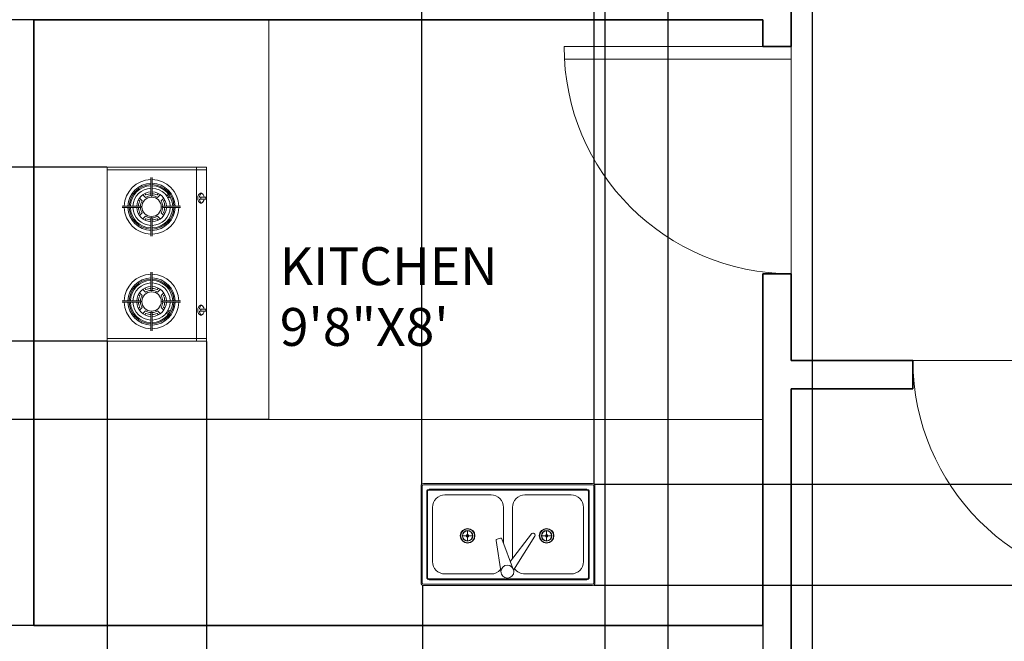
# Model space of a CAD drawing. Units: inches. Extents: x -438 to 102, y -60 to 1091.
# Tile 9 of 20: x -305 to -149, y 799 to 898. Entities that reach past the tile are written whole.
import ezdxf

# ---------------------------------------------------------------- set-up
doc = ezdxf.new("R2010")
doc.units = ezdxf.units.IN
doc.header["$MEASUREMENT"] = 0
for name, color, linetype, lineweight, true_color in [('A-ANNO-DIMS', 217, 'Continuous', 18, 0x93278f), ('A-DOOR', 30, 'Continuous', 18, 0xf26722), ('A-WALL', 2, 'Continuous', 35, 0xf1eb1f)]:
    doc.layers.add(name, color=color, linetype=linetype, lineweight=lineweight, true_color=true_color)
for name, color, linetype, lineweight in [('A-AREA-IDEN', 4, 'Continuous', 18), ('A-EQPM', 9, 'Continuous', 15), ('A-FLOR-CASE', 7, 'Continuous', 18), ('A-FLOR-FIXT', 9, 'Continuous', 15)]:
    doc.layers.add(name, color=color, linetype=linetype, lineweight=lineweight)
doc.styles.get("Standard").update_dxf_attribs({"font": 'arial.ttf'})
doc.dimstyles.get("Standard").update_dxf_attribs({"dimtxt": 8, "dimasz": 0.18, "dimexe": 0.18, "dimexo": 0.0625, "dimgap": 0.09, "dimtad": 0, "dimtih": 1, "dimtoh": 1, "dimdec": 4, "dimzin": 0, "dimdsep": 46, "dimlunit": 3, "dimtxsty": 'Standard', "dimcen": 0.09, "dimadec": 0, "dimazin": 0, "dimtfac": 1, "dimtdec": 4, "dimtofl": 0, "dimtmove": 0, "dimatfit": 3, "dimfxl": 1, "dimtolj": 1, "dimtzin": 0, "dimarcsym": 0})

# ---------------------------------------------------------------- blocks, each defined once
blk = doc.blocks.new('DOOR-SWING-36')
for p, q in [((-36, 0), (0, 0)), ((-2, 0), (-2, -36)), ((0, 0), (0, -36))]:
    blk.add_line(p, q)
blk.add_arc((0, 0), 36, 180, 270)
blk = doc.blocks.new('*D37')
at = {"layer": 'A-ANNO-DIMS', "color": 0, "lineweight": -2, "transparency": 16777216}
for p, q in [((-179.8, 234.94), (-179.8, 1079.58)), ((-134.08, 234.94), (-134.08, 1079.58)), ((-179.62, 1079.4), (-176.98, 1079.4)), ((-134.26, 1079.4), (-136.9, 1079.4))]:
    blk.add_line(p, q, dxfattribs=at)
at = {"layer": 'A-ANNO-DIMS', "color": 0, "transparency": 16777216}
for points in [[(-179.62, 1079.43), (-179.62, 1079.37), (-179.8, 1079.4)], [(-134.26, 1079.43), (-134.26, 1079.37), (-134.08, 1079.4)]]:
    blk.add_solid(points, dxfattribs=at)
at = {"layer": 'Defpoints', "color": 0, "transparency": 16777216}
for p in [(-134.08, 1079.4), (-179.8, 234.88), (-134.08, 234.88)]:
    blk.add_point(p, dxfattribs=at)
at = {"layer": 'A-ANNO-DIMS', "color": 0, "transparency": 16777216, "insert": (-156.94, 1079.4), "char_height": 8, "attachment_point": 5}
blk.add_mtext('\\A1;3\'-9 1/2"', dxfattribs=at)
blk = doc.blocks.new('*D42')
at = {"layer": 'A-ANNO-DIMS', "color": 0, "lineweight": -2, "transparency": 16777216}
for p, q in [((-266, 834.64), (-414.94, 834.64)), ((-414.76, 834.46), (-414.76, 822.55)), ((-414.76, 802.18), (-414.76, 814.09)), ((-303.21, 802), (-414.94, 802))]:
    blk.add_line(p, q, dxfattribs=at)
at = {"layer": 'A-ANNO-DIMS', "color": 0, "transparency": 16777216}
for points in [[(-414.79, 834.46), (-414.73, 834.46), (-414.76, 834.64)], [(-414.79, 802.18), (-414.73, 802.18), (-414.76, 802)]]:
    blk.add_solid(points, dxfattribs=at)
at = {"layer": 'Defpoints', "color": 0, "transparency": 16777216}
for p in [(-414.76, 834.64), (-265.94, 834.64), (-303.15, 802)]:
    blk.add_point(p, dxfattribs=at)
at = {"layer": 'A-ANNO-DIMS', "color": 0, "transparency": 16777216, "insert": (-414.76, 818.32), "char_height": 8, "attachment_point": 5}
blk.add_mtext('\\A1;2\'-8 1/2"', dxfattribs=at)
blk = doc.blocks.new('*D51')
at = {"layer": 'A-ANNO-DIMS', "color": 0, "lineweight": -2, "transparency": 16777216}
for p, q in [((-291.54, 847), (-291.54, -48.58)), ((-275.79, 847), (-275.79, -48.58)), ((-291.36, -48.4), (-275.97, -48.4)), ((-275.79, -48.4), (-275.61, -48.4))]:
    blk.add_line(p, q, dxfattribs=at)
at = {"layer": 'A-ANNO-DIMS', "color": 0, "transparency": 16777216}
for points in [[(-291.36, -48.37), (-291.36, -48.43), (-291.54, -48.4)], [(-275.97, -48.37), (-275.97, -48.43), (-275.79, -48.4)]]:
    blk.add_solid(points, dxfattribs=at)
at = {"layer": 'Defpoints', "color": 0, "transparency": 16777216}
for p in [(-291.54, 847.06), (-275.79, 847.06), (-275.79, -48.4)]:
    blk.add_point(p, dxfattribs=at)
at = {"layer": 'A-ANNO-DIMS', "color": 0, "transparency": 16777216, "insert": (-255.95, -48.4), "char_height": 8, "attachment_point": 5}
blk.add_mtext('\\A1;1\'-3 1/2"', dxfattribs=at)
blk = doc.blocks.new('*D52')
at = {"layer": 'A-ANNO-DIMS', "color": 0, "lineweight": -2, "transparency": 16777216}
for p, q in [((-291.6, 874.62), (-414.94, 874.62)), ((-414.76, 874.44), (-414.76, 865.07)), ((-414.76, 847.24), (-414.76, 856.61)), ((-291.6, 847.06), (-414.94, 847.06))]:
    blk.add_line(p, q, dxfattribs=at)
at = {"layer": 'A-ANNO-DIMS', "color": 0, "transparency": 16777216}
for points in [[(-414.79, 874.44), (-414.73, 874.44), (-414.76, 874.62)], [(-414.79, 847.24), (-414.73, 847.24), (-414.76, 847.06)]]:
    blk.add_solid(points, dxfattribs=at)
at = {"layer": 'Defpoints', "color": 0, "transparency": 16777216}
for p in [(-414.76, 874.62), (-291.54, 874.62), (-291.54, 847.06)]:
    blk.add_point(p, dxfattribs=at)
at = {"layer": 'A-ANNO-DIMS', "color": 0, "transparency": 16777216, "insert": (-414.76, 860.84), "char_height": 8, "attachment_point": 5}
blk.add_mtext('\\A1;2\'-3 1/2"', dxfattribs=at)
blk = doc.blocks.new('*D53')
at = {"layer": 'A-ANNO-DIMS', "color": 0, "lineweight": -2, "transparency": 16777216}
for p, q in [((-241.7, 824.44), (-241.7, 1079.58)), ((-214.37, 824.44), (-214.37, 1079.58)), ((-241.52, 1079.4), (-214.55, 1079.4)), ((-214.37, 1079.4), (-214.19, 1079.4))]:
    blk.add_line(p, q, dxfattribs=at)
at = {"layer": 'A-ANNO-DIMS', "color": 0, "transparency": 16777216}
for points in [[(-241.52, 1079.43), (-241.52, 1079.37), (-241.7, 1079.4)], [(-214.55, 1079.43), (-214.55, 1079.37), (-214.37, 1079.4)]]:
    blk.add_solid(points, dxfattribs=at)
at = {"layer": 'Defpoints', "color": 0, "transparency": 16777216}
for p in [(-214.37, 1079.4), (-241.7, 824.38), (-214.37, 824.38)]:
    blk.add_point(p, dxfattribs=at)
at = {"layer": 'A-ANNO-DIMS', "color": 0, "transparency": 16777216, "insert": (-194.08, 1079.4), "char_height": 8, "attachment_point": 5}
blk.add_mtext('\\A1;2\'-3 1/2"', dxfattribs=at)
blk = doc.blocks.new('*D54')
at = {"layer": 'A-ANNO-DIMS', "color": 0, "lineweight": -2, "transparency": 16777216}
for p, q in [((-214.3, 824.38), (81.43, 824.38)), ((81.25, 824.2), (81.25, 820.49)), ((81.25, 808.56), (81.25, 812.28)), ((-214.43, 808.38), (81.43, 808.38))]:
    blk.add_line(p, q, dxfattribs=at)
at = {"layer": 'A-ANNO-DIMS', "color": 0, "transparency": 16777216}
for points in [[(81.22, 824.2), (81.28, 824.2), (81.25, 824.38)], [(81.22, 808.56), (81.28, 808.56), (81.25, 808.38)]]:
    blk.add_solid(points, dxfattribs=at)
at = {"layer": 'Defpoints', "color": 0, "transparency": 16777216}
for p in [(-214.37, 824.38), (81.25, 824.38), (-214.49, 808.38)]:
    blk.add_point(p, dxfattribs=at)
at = {"layer": 'A-ANNO-DIMS', "color": 0, "transparency": 16777216, "insert": (81.25, 816.38), "char_height": 8, "attachment_point": 5}
blk.add_mtext('\\A1;1\'-4"', dxfattribs=at)
blk = doc.blocks.new('*D55')
at = {"layer": 'A-ANNO-DIMS', "color": 0, "lineweight": -2, "transparency": 16777216}
for p, q in [((-241.57, 808.32), (-241.57, -48.58)), ((-187.65, 801.94), (-187.65, -48.58)), ((-241.39, -48.4), (-225.49, -48.4)), ((-187.83, -48.4), (-203.72, -48.4))]:
    blk.add_line(p, q, dxfattribs=at)
at = {"layer": 'A-ANNO-DIMS', "color": 0, "transparency": 16777216}
for points in [[(-241.39, -48.37), (-241.39, -48.43), (-241.57, -48.4)], [(-187.83, -48.37), (-187.83, -48.43), (-187.65, -48.4)]]:
    blk.add_solid(points, dxfattribs=at)
at = {"layer": 'Defpoints', "color": 0, "transparency": 16777216}
for p in [(-241.57, 808.38), (-187.65, 802), (-187.65, -48.4)]:
    blk.add_point(p, dxfattribs=at)
at = {"layer": 'A-ANNO-DIMS', "color": 0, "transparency": 16777216, "insert": (-214.61, -48.4), "char_height": 8, "attachment_point": 5}
blk.add_mtext('\\A1;4\'-6"', dxfattribs=at)
blk = doc.blocks.new('*D56')
at = {"layer": 'A-ANNO-DIMS', "color": 0, "lineweight": -2, "transparency": 16777216}
for p, q in [((-303.21, 898), (-414.94, 898)), ((-414.76, 897.82), (-414.76, 890.54)), ((-414.76, 874.8), (-414.76, 882.08)), ((-291.6, 874.62), (-414.94, 874.62))]:
    blk.add_line(p, q, dxfattribs=at)
at = {"layer": 'A-ANNO-DIMS', "color": 0, "transparency": 16777216}
for points in [[(-414.79, 897.82), (-414.73, 897.82), (-414.76, 898)], [(-414.79, 874.8), (-414.73, 874.8), (-414.76, 874.62)]]:
    blk.add_solid(points, dxfattribs=at)
at = {"layer": 'Defpoints', "color": 0, "transparency": 16777216}
for p in [(-414.76, 898), (-303.15, 898), (-291.54, 874.62)]:
    blk.add_point(p, dxfattribs=at)
at = {"layer": 'A-ANNO-DIMS', "color": 0, "transparency": 16777216, "insert": (-414.76, 886.31), "char_height": 8, "attachment_point": 5}
blk.add_mtext('\\A1;1\'-11 1/2"', dxfattribs=at)
blk = doc.blocks.new('*D61')
at = {"layer": 'A-ANNO-DIMS', "color": 0, "lineweight": -2, "transparency": 16777216}
for p, q in [((-212.65, 534.56), (-212.65, 1079.58)), ((-202.65, 534.56), (-202.65, 1079.58)), ((-212.65, 1079.4), (-212.83, 1079.4)), ((-202.83, 1079.4), (-212.47, 1079.4))]:
    blk.add_line(p, q, dxfattribs=at)
at = {"layer": 'A-ANNO-DIMS', "color": 0, "transparency": 16777216}
for points in [[(-212.47, 1079.43), (-212.47, 1079.37), (-212.65, 1079.4)], [(-202.83, 1079.43), (-202.83, 1079.37), (-202.65, 1079.4)]]:
    blk.add_solid(points, dxfattribs=at)
at = {"layer": 'Defpoints', "color": 0, "transparency": 16777216}
for p in [(-212.65, 1079.4), (-212.65, 534.5), (-202.65, 534.5)]:
    blk.add_point(p, dxfattribs=at)
at = {"layer": 'A-ANNO-DIMS', "color": 0, "transparency": 16777216, "insert": (-226.66, 1079.4), "char_height": 8, "attachment_point": 5}
blk.add_mtext('\\A1;0\'-10"', dxfattribs=at)

msp = doc.modelspace()

# ---------------------------------------------------------------- linework, layer by layer
at = {"layer": 'A-EQPM'}
for p, q in [((-275.79225, 874.62295), (-291.54025, 874.62295)), ((-291.54025, 874.62295), (-291.54025, 847.06395)), ((-275.79225, 874.22925), (-291.54025, 874.22925)), ((-277.36705, 847.06395), (-277.36705, 874.62295)), ((-275.79225, 847.06395), (-275.79225, 874.62295)), ((-284.59767, 870.11341), (-284.59767, 872.9792)), ((-284.40082, 870.11341), (-284.40082, 872.9792)), ((-276.61681, 870.50215), (-276.7582, 870.50215)), ((-286.3881, 869.23116), (-286.59373, 869.43679)), ((-285.99905, 869.28753), (-286.4246, 869.71307)), ((-285.44228, 869.84431), (-285.86782, 870.26985)), ((-285.3859, 870.23335), (-285.59154, 870.43899)), ((-283.40695, 870.43899), (-283.61258, 870.23335)), ((-283.13067, 870.26985), (-283.55621, 869.84431)), ((-282.57389, 869.71307), (-282.99943, 869.28753)), ((-282.40475, 869.43679), (-282.61039, 869.23116)), ((-276.62233, 869.89058), (-276.84294, 869.89058)), ((-276.62233, 869.54023), (-276.83821, 869.54023)), ((-276.61681, 868.94788), (-276.7582, 868.94788)), ((-276.70107, 869.81184), (-276.70107, 869.61897)), ((-275.95827, 869.89058), (-276.62233, 869.89058)), ((-276.62233, 869.54023), (-275.95827, 869.54023)), ((-275.87953, 869.61897), (-275.87953, 869.81184)), ((-286.26816, 868.44292), (-289.18049, 868.44292)), ((-286.26816, 868.24607), (-289.18049, 868.24607)), ((-286.3881, 867.45784), (-286.59373, 867.2522)), ((-285.99905, 867.40146), (-286.4246, 866.97592)), ((-282.57389, 866.97592), (-282.99943, 867.40146)), ((-282.73033, 868.44292), (-279.89669, 868.44292)), ((-282.73033, 868.24607), (-279.89669, 868.24607)), ((-282.40475, 867.2522), (-282.61039, 867.45784)), ((-285.44228, 866.84469), (-285.86782, 866.41914)), ((-285.3859, 866.45564), (-285.59154, 866.25001)), ((-284.59767, 866.57558), (-284.59767, 863.67981)), ((-284.40082, 866.57558), (-284.40082, 863.67981)), ((-283.40695, 866.25001), (-283.61258, 866.45564)), ((-283.13067, 866.41914), (-283.55621, 866.84469)), ((-284.59767, 855.11132), (-284.59767, 858.00709)), ((-284.40082, 855.11132), (-284.40082, 858.00709)), ((-285.44228, 854.84222), (-285.86782, 855.26776)), ((-285.3859, 855.23126), (-285.59154, 855.4369)), ((-283.40695, 855.4369), (-283.61258, 855.23126)), ((-283.13067, 855.26776), (-283.55621, 854.84222)), ((-286.26816, 853.44083), (-289.18049, 853.44083)), ((-286.3881, 854.22907), (-286.59373, 854.4347)), ((-285.99905, 854.28544), (-286.4246, 854.71098)), ((-282.57389, 854.71098), (-282.99943, 854.28544)), ((-282.73033, 853.44083), (-279.89669, 853.44083)), ((-282.40475, 854.4347), (-282.61039, 854.22907)), ((-286.26816, 853.24398), (-289.18049, 853.24398)), ((-286.3881, 852.45575), (-286.59373, 852.25011)), ((-285.99905, 852.39937), (-286.4246, 851.97383)), ((-285.44228, 851.8426), (-285.86782, 851.41705)), ((-283.13067, 851.41705), (-283.55621, 851.8426)), ((-282.57389, 851.97383), (-282.99943, 852.39937)), ((-282.73033, 853.24398), (-279.89669, 853.24398)), ((-282.40475, 852.25011), (-282.61039, 852.45575)), ((-276.62233, 851.79632), (-276.84294, 851.79632)), ((-276.62233, 852.14668), (-276.83821, 852.14668)), ((-276.61681, 852.73903), (-276.7582, 852.73903)), ((-276.70107, 851.87506), (-276.70107, 852.06794)), ((-276.62233, 852.14668), (-275.95827, 852.14668)), ((-275.95827, 851.79632), (-276.62233, 851.79632)), ((-275.87953, 852.06794), (-275.87953, 851.87506)), ((-285.3859, 851.45355), (-285.59154, 851.24792)), ((-284.59767, 851.57349), (-284.59767, 848.70771)), ((-284.40082, 851.57349), (-284.40082, 848.70771)), ((-283.40695, 851.24792), (-283.61258, 851.45355)), ((-276.61681, 851.18475), (-276.7582, 851.18475)), ((-291.54025, 847.45765), (-275.79225, 847.45765)), ((-291.54025, 847.06395), (-275.79225, 847.06395))]:
    msp.add_line(p, q, dxfattribs=at)
for centre, radius in [((-284.49924, 868.3445), 1.53543), ((-281.94866, 870.25782), 0.14088), ((-281.71748, 869.90086), 0.14088), ((-284.49924, 853.34241), 1.53543), ((-281.71748, 851.78604), 0.14088), ((-281.94866, 851.42908), 0.14088)]:
    msp.add_circle(centre, radius, dxfattribs=at)
for centre, radius, start, end in [((-284.49924, 868.3445), 4.3307, 91.3022889, 178.6977111), ((-284.49924, 868.3445), 3.74015, 91.5917542, 178.4082458), ((-284.49924, 868.3445), 4.3307, 1.3022889, 88.6977111), ((-284.49924, 868.3445), 3.74015, 1.5917542, 88.4082458), ((-284.49924, 868.3445), 3.5433, 91.5917542, 178.4082458), ((-284.49924, 868.3445), 3.34645, 91.685413, 178.314587), ((-284.49924, 868.3445), 2.95275, 91.9102132, 178.0897868), ((-284.49924, 868.3445), 2.3622, 92.3880155, 177.6119845), ((-284.49924, 868.3445), 3.5433, 1.5917542, 88.4082458), ((-284.49924, 868.3445), 3.34645, 1.685413, 88.314587), ((-284.49924, 868.3445), 2.95275, 1.9102132, 88.0897868), ((-284.49924, 868.3445), 2.3622, 2.3880155, 87.6119845), ((-275.81005, 869.72501), 1.14013, 138.6513888, 166.6924973), ((-276.60684, 870.42621), 0.07874, 75.3271166, 138.6513888), ((-284.49924, 868.3445), 2.08661, 154.853885, 177.2963657), ((-284.49924, 868.3445), 1.77165, 147.8395884, 176.8152615), ((-284.49924, 868.3445), 1.77165, 93.1847385, 122.1604116), ((-284.49924, 868.3445), 2.08661, 92.7036343, 115.146115), ((-284.49924, 870.12503), 0.09911, 186.7353744, 353.2646256), ((-284.49924, 868.3445), 2.08661, 64.853885, 87.2963657), ((-284.49924, 868.3445), 1.77165, 57.8395884, 86.8152615), ((-284.49924, 868.3445), 1.77165, 3.1847385, 32.1604116), ((-284.49924, 868.3445), 2.08661, 2.7036343, 25.146115), ((-276.84294, 869.96932), 0.07874, 166.6924973, 270), ((-276.83821, 869.46149), 0.07874, 90, 194.3759834), ((-275.81005, 869.72501), 1.14013, 194.3759834, 219.6110848), ((-276.62233, 869.81184), 0.07874, 90, 180), ((-276.62233, 869.61897), 0.07874, 180, 270), ((-276.59844, 869.05019), 0.10396, 210.0749159, 302.1858261), ((-275.95827, 869.81184), 0.07874, 0, 90), ((-275.95827, 869.61897), 0.07874, 270, 0), ((-284.49924, 868.3445), 4.3307, 181.3022889, 268.6977111), ((-284.49924, 868.3445), 3.74015, 181.5917542, 268.4082458), ((-284.49924, 868.3445), 3.5433, 181.5917542, 268.4082458), ((-284.49924, 868.3445), 3.34645, 181.685413, 268.314587), ((-284.49924, 868.3445), 2.95275, 181.9102132, 268.0897868), ((-284.49924, 868.3445), 2.3622, 182.3880155, 267.6119845), ((-284.49924, 868.3445), 2.08661, 182.7036343, 205.146115), ((-286.30506, 868.3445), 0.10511, 290.550693, 69.449307), ((-284.49924, 868.3445), 1.77165, 183.1847385, 212.1604116), ((-284.49924, 868.3445), 2.3622, 272.3880155, 357.6119845), ((-284.49924, 868.3445), 4.3307, 271.3022889, 358.6977111), ((-284.49924, 868.3445), 3.34645, 271.685413, 358.314587), ((-284.49924, 868.3445), 2.95275, 271.9102132, 358.0897868), ((-284.49924, 868.3445), 3.5433, 271.5917542, 358.4082458), ((-284.49924, 868.3445), 3.74015, 271.5917542, 358.4082458), ((-284.49924, 868.3445), 1.77165, 327.8395884, 356.8152615), ((-282.69692, 868.3445), 0.10394, 108.751046, 251.248954), ((-284.49924, 868.3445), 2.08661, 334.853885, 357.2963657), ((-284.49924, 868.3445), 1.77165, 237.8395884, 266.8152615), ((-284.49924, 868.3445), 2.08661, 244.853885, 267.2963657), ((-284.49924, 866.53624), 0.106, 21.7885229, 158.2114771), ((-284.49924, 868.3445), 1.77165, 273.1847385, 302.1604116), ((-284.49924, 868.3445), 2.08661, 272.7036343, 295.146115), ((-284.49924, 853.34241), 4.3307, 91.3022889, 178.6977111), ((-284.49924, 853.34241), 3.74015, 91.5917542, 178.4082458), ((-284.49924, 853.34241), 3.5433, 91.5917542, 178.4082458), ((-284.49924, 853.34241), 3.34645, 91.685413, 178.314587), ((-284.49924, 853.34241), 4.3307, 1.3022889, 88.6977111), ((-284.49924, 853.34241), 3.5433, 1.5917542, 88.4082458), ((-284.49924, 853.34241), 3.34645, 1.685413, 88.314587), ((-284.49924, 853.34241), 3.74015, 1.5917542, 88.4082458), ((-284.49924, 853.34241), 2.95275, 91.9102132, 178.0897868), ((-284.49924, 853.34241), 2.3622, 92.3880155, 177.6119845), ((-284.49924, 853.34241), 1.77165, 93.1847385, 122.1604116), ((-284.49924, 853.34241), 2.08661, 92.7036343, 115.146115), ((-284.49924, 855.15066), 0.106, 201.7885229, 338.2114771), ((-284.49924, 853.34241), 2.95275, 1.9102132, 88.0897868), ((-284.49924, 853.34241), 2.3622, 2.3880155, 87.6119845), ((-284.49924, 853.34241), 2.08661, 64.853885, 87.2963657), ((-284.49924, 853.34241), 1.77165, 57.8395884, 86.8152615), ((-284.49924, 853.34241), 2.08661, 154.853885, 177.2963657), ((-284.49924, 853.34241), 1.77165, 147.8395884, 176.8152615), ((-286.30506, 853.34241), 0.10511, 290.550693, 69.449307), ((-284.49924, 853.34241), 1.77165, 3.1847385, 32.1604116), ((-282.69692, 853.34241), 0.10394, 108.751046, 251.248954), ((-284.49924, 853.34241), 2.08661, 2.7036343, 25.146115), ((-284.49924, 853.34241), 4.3307, 181.3022889, 268.6977111), ((-284.49924, 853.34241), 3.74015, 181.5917542, 268.4082458), ((-284.49924, 853.34241), 3.5433, 181.5917542, 268.4082458), ((-284.49924, 853.34241), 3.34645, 181.685413, 268.314587), ((-284.49924, 853.34241), 2.95275, 181.9102132, 268.0897868), ((-284.49924, 853.34241), 2.3622, 182.3880155, 267.6119845), ((-284.49924, 853.34241), 2.08661, 182.7036343, 205.146115), ((-284.49924, 853.34241), 1.77165, 183.1847385, 212.1604116), ((-284.49924, 853.34241), 1.77165, 237.8395884, 266.8152615), ((-284.49924, 853.34241), 2.3622, 272.3880155, 357.6119845), ((-284.49924, 853.34241), 4.3307, 271.3022889, 358.6977111), ((-284.49924, 853.34241), 2.95275, 271.9102132, 358.0897868), ((-284.49924, 853.34241), 3.34645, 271.685413, 358.314587), ((-284.49924, 853.34241), 3.5433, 271.5917542, 358.4082458), ((-284.49924, 853.34241), 1.77165, 273.1847385, 302.1604116), ((-284.49924, 853.34241), 3.74015, 271.5917542, 358.4082458), ((-284.49924, 853.34241), 1.77165, 327.8395884, 356.8152615), ((-284.49924, 853.34241), 2.08661, 334.853885, 357.2963657), ((-276.84294, 851.71758), 0.07874, 90, 193.3075027), ((-276.83821, 852.22542), 0.07874, 165.6240166, 270), ((-275.81005, 851.96189), 1.14013, 140.3889152, 165.6240166), ((-276.62233, 852.06794), 0.07874, 90, 180), ((-276.62233, 851.87506), 0.07874, 180, 270), ((-276.59844, 852.63671), 0.10396, 57.8141739, 149.9250841), ((-275.95827, 852.06794), 0.07874, 0, 90), ((-275.95827, 851.87506), 0.07874, 270, 0), ((-284.49924, 853.34241), 2.08661, 244.853885, 267.2963657), ((-284.49924, 851.56187), 0.09911, 6.7353744, 173.2646256), ((-284.49924, 853.34241), 2.08661, 272.7036343, 295.146115), ((-275.81005, 851.96189), 1.14013, 193.3075027, 221.3486112), ((-276.60684, 851.2607), 0.07874, 221.3486112, 284.6728834)]:
    msp.add_arc(centre, radius, start, end, dxfattribs=at)
at = {"layer": 'A-EQPM', "extrusion": (0, 0, -1)}
for start_param, end_param in [(3.311146783, 6.113631178), (0.167831346, 1.359229349), (1.807363774, 2.885845936)]:
    msp.add_ellipse((-276.67212, 869.72501), major_axis=(0, 0.78844), ratio=0.64705753, start_param=start_param, end_param=end_param, dxfattribs=at)
at = {"layer": 'A-EQPM'}
for start_param, end_param in [(3.311146783, 6.113631178), (0.167831346, 1.359229349), (1.807363774, 2.885845936)]:
    msp.add_ellipse((-276.67212, 851.96189), major_axis=(0, -0.78844), ratio=0.64705753, start_param=start_param, end_param=end_param, dxfattribs=at)
at = {"layer": 'A-FLOR-CASE'}
for p, q in [((-265.93641, 897.99939), (-265.93641, 834.64014)), ((-265.93641, 834.64014), (-187.64649, 834.64014))]:
    msp.add_line(p, q, dxfattribs=at)
at = {"layer": 'A-FLOR-FIXT'}
for p, q in [((-241.81089, 824.101), (-241.81089, 808.7467)), ((-241.61404, 824.101), (-241.61404, 808.7467)), ((-214.64559, 824.4947), (-241.41719, 824.4947)), ((-214.64559, 824.29785), (-241.41719, 824.29785)), ((-214.44874, 808.7467), (-214.44874, 824.101)), ((-214.25189, 808.7467), (-214.25189, 824.101)), ((-240.90538, 823.19549), (-240.90538, 809.65221)), ((-240.78727, 823.19549), (-240.78727, 809.65221)), ((-215.5511, 823.58919), (-240.51168, 823.58919)), ((-215.5511, 823.47108), (-240.51168, 823.47108)), ((-230.70855, 822.68368), (-238.03137, 822.68368)), ((-218.03141, 822.68368), (-225.35423, 822.68368)), ((-215.27551, 809.65221), (-215.27551, 823.19549)), ((-215.1574, 809.65221), (-215.1574, 823.19549)), ((-239.99987, 820.71518), (-239.99987, 812.13252)), ((-228.74005, 815.05351), (-228.74005, 820.71518)), ((-227.32273, 820.71518), (-227.32273, 812.61996)), ((-216.06291, 812.13252), (-216.06291, 820.71518)), ((-234.63258, 816.21228), (-235.22307, 816.21228)), ((-234.42871, 816.41615), (-234.42871, 817.00665)), ((-234.42871, 816.00841), (-234.42871, 815.41791)), ((-234.22484, 816.21228), (-233.63434, 816.21228)), ((-227.6585, 812.18367), (-224.3256, 816.51442)), ((-227.13372, 810.79119), (-223.78431, 816.13685)), ((-223.88923, 816.57594), (-223.86444, 816.55768)), ((-222.11493, 816.21228), (-222.70543, 816.21228)), ((-221.91106, 816.41615), (-221.91106, 817.00665)), ((-221.91106, 816.00841), (-221.91106, 815.41791)), ((-221.70719, 816.21228), (-221.1167, 816.21228)), ((-229.91661, 815.47446), (-229.12216, 810.28179)), ((-229.2218, 815.83512), (-229.77073, 815.69496)), ((-227.13372, 810.79119), (-228.98889, 815.71381)), ((-238.03137, 810.16402), (-230.70855, 810.16402)), ((-225.35423, 810.16402), (-218.03141, 810.16402)), ((-241.41719, 808.54985), (-214.64559, 808.54985)), ((-241.41719, 808.353), (-214.64559, 808.353)), ((-240.51168, 809.37662), (-215.5511, 809.37662)), ((-240.51168, 809.25851), (-215.5511, 809.25851))]:
    msp.add_line(p, q, dxfattribs=at)
for centre, radius in [((-234.42871, 816.21228), 1.16204), ((-234.42871, 816.21228), 1.09933), ((-234.42871, 816.21228), 0.83003), ((-234.42871, 816.21228), 0.79437), ((-234.42871, 816.21228), 0.20387), ((-234.42871, 816.21228), 0.09579), ((-221.91106, 816.21228), 1.16204), ((-221.91106, 816.21228), 1.09933), ((-221.91106, 816.21228), 0.83003), ((-221.91106, 816.21228), 0.79437), ((-221.91106, 816.21228), 0.20387), ((-221.91106, 816.21228), 0.09579), ((-228.12794, 810.53649), 1.02633)]:
    msp.add_circle(centre, radius, dxfattribs=at)
for centre, radius, start, end in [((-241.41719, 824.101), 0.3937, 90, 180), ((-241.41719, 824.101), 0.19685, 90, 180), ((-214.64559, 824.101), 0.3937, 0, 90), ((-214.64559, 824.101), 0.19685, 0, 90), ((-240.51168, 823.19549), 0.3937, 90, 180), ((-240.51168, 823.19549), 0.27559, 90, 180), ((-238.03137, 820.71518), 1.9685, 90, 180), ((-230.70855, 820.71518), 1.9685, 0, 90), ((-225.35423, 820.71518), 1.9685, 90, 180), ((-218.03141, 820.71518), 1.9685, 0, 90), ((-215.5511, 823.19549), 0.3937, 0, 90), ((-215.5511, 823.19549), 0.27559, 0, 90), ((-224.076, 816.32233), 0.31496, 53.6309311, 142.4185447), ((-224.05121, 816.30407), 0.31496, 327.9301426, 53.6309311), ((-229.72203, 815.50423), 0.19685, 104.3233276, 188.6985351), ((-229.1731, 815.64439), 0.19685, 20.6498216, 104.3233276), ((-238.03137, 812.13252), 1.9685, 180, 270), ((-218.03141, 812.13252), 1.9685, 270, 0), ((-240.51168, 809.65221), 0.3937, 180, 270), ((-240.51168, 809.65221), 0.27559, 180, 270), ((-230.70855, 812.13252), 1.9685, 270, 319.5750097), ((-225.35423, 812.13252), 1.9685, 214.0864438, 270), ((-215.5511, 809.65221), 0.27559, 270, 0), ((-215.5511, 809.65221), 0.3937, 270, 0), ((-241.41719, 808.7467), 0.3937, 180, 270), ((-241.41719, 808.7467), 0.19685, 180, 270), ((-214.64559, 808.7467), 0.19685, 270, 0), ((-214.64559, 808.7467), 0.3937, 270, 0)]:
    msp.add_arc(centre, radius, start, end, dxfattribs=at)
at = {"layer": 'A-WALL'}
for p, q in [((-183.14649, 907.50091), (-183.14649, 893.74862)), ((-187.64649, 897.99939), (-303.14649, 897.99939)), ((-303.14649, 897.99939), (-303.14649, 801.99939)), ((-187.64649, 897.99939), (-187.64649, 893.74862)), ((-183.14649, 893.74862), (-187.64649, 893.74862)), ((-183.14649, 857.74862), (-187.64649, 857.74862)), ((-187.64649, 857.74862), (-187.64649, 801.99939)), ((-183.14649, 857.74862), (-183.14649, 843.99939)), ((-163.87208, 843.99939), (-183.14649, 843.99939)), ((-163.87208, 839.49939), (-163.87208, 843.99939)), ((-183.14649, 839.49939), (-183.14649, 797.49939)), ((-163.87208, 839.49939), (-183.14649, 839.49939)), ((-187.64649, 801.99939), (-303.14649, 801.99939))]:
    msp.add_line(p, q, dxfattribs=at)

# ---------------------------------------------------------------- block references
at = {"layer": 'A-DOOR', "extrusion": (0, 0, -1), "zscale": -1, "rotation": 89.99999999999982}
msp.add_blockref('DOOR-SWING-36', (183.14649, 893.74862), dxfattribs=at)
at = {"layer": 'A-DOOR'}
msp.add_blockref('DOOR-SWING-36', (-127.87208, 843.99939), dxfattribs=at)

# ---------------------------------------------------------------- texts
at = {"layer": 'A-AREA-IDEN'}
for s, p in [('KITCHEN', (-264.18552, 855.9475)), ('9\'8"X8\'', (-264.18552, 846.30903))]:
    msp.add_text(s, height=6, dxfattribs=at).set_placement(p)

# ---------------------------------------------------------------- dimensions: what is measured, and where the dimension line sits
at = {"layer": 'A-ANNO-DIMS'}
for base, p1, p2, picture, middle in [((-214.3672, 1079.39939), (-241.69558, 824.37939), (-214.3672, 824.37939), '*D53', (-194.07537, 1079.39939)), ((-134.07948, 1079.39939), (-179.79585, 234.87846), (-134.07948, 234.87846), '*D37', (-156.93767, 1079.39939)), ((-212.64649, 1079.39939), (-202.64649, 534.49939), (-212.64649, 534.49939), '*D61', (-226.65728, 1079.39939)), ((-275.79225, -48.40061), (-291.54025, 847.06395), (-275.79225, 847.06395), '*D51', (-255.94517, -48.40061)), ((-187.64649, -48.40061), (-241.57044, 808.38394), (-187.64649, 801.99939), '*D55', (-214.60846, -48.40061))]:
    dim = msp.add_linear_dim(base=base, p1=p1, p2=p2, dimstyle='Standard', override={"dimdec": 1, "dimlfac": 1, "dimrnd": 0, "dimzin": 1, "dimdsep": 46, "dimlunit": 4, "dimfrac": 2}, dxfattribs=at)
    dim.commit()
    dim.dimension.update_dxf_attribs({"geometry": picture, "text_midpoint": middle})
for base, p1, p2, picture, middle in [((-414.76009, 897.99939), (-291.54025, 874.62295), (-303.14649, 897.99939), '*D56', (-414.76009, 886.31117)), ((-414.76009, 874.62295), (-291.54025, 847.06395), (-291.54025, 874.62295), '*D52', (-414.76009, 860.84345)), ((-414.76009, 834.64014), (-303.14649, 801.99939), (-265.93641, 834.64014), '*D42', (-414.76009, 818.31976)), ((81.25351, 824.37939), (-214.49234, 808.38394), (-214.3672, 824.37939), '*D54', (81.25351, 816.38167))]:
    dim = msp.add_linear_dim(base=base, p1=p1, p2=p2, angle=90, dimstyle='Standard', override={"dimdec": 1, "dimlfac": 1, "dimrnd": 0, "dimzin": 1, "dimdsep": 46, "dimlunit": 4, "dimfrac": 2}, dxfattribs=at)
    dim.commit()
    dim.dimension.update_dxf_attribs({"geometry": picture, "text_midpoint": middle})

doc.saveas('drawing.dxf')
